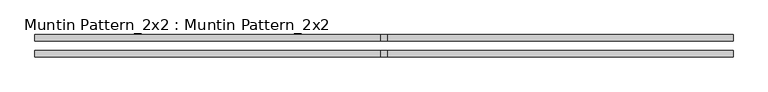
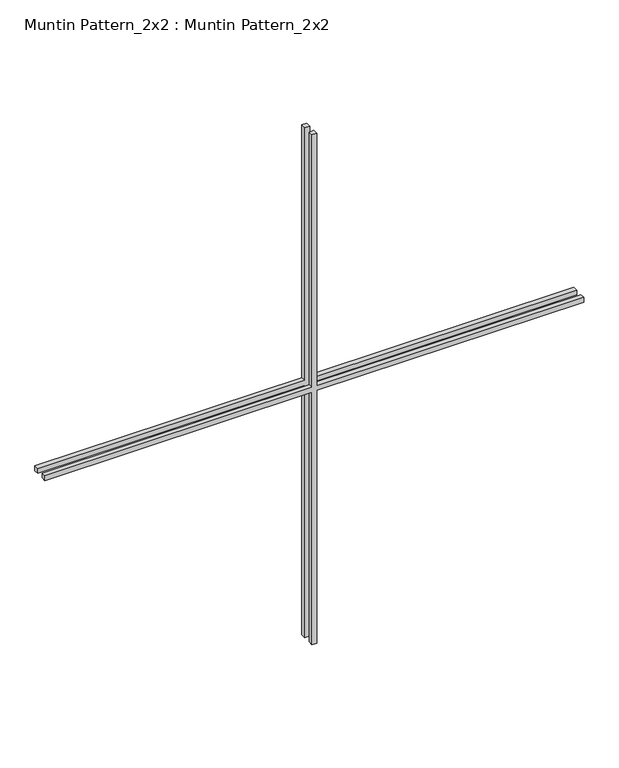
"""IFC4 building model written with IfcOpenShell, lengths in millimetres: proxy geometry, Muntin Pattern_2x2 : Muntin Pattern_2x2."""

from ifc_helpers import new_model, si_unit, frame, origin, place, context, project, spatial, polyline, outline, extrude, source, transform, mapped, element, save


def muntin_pattern_2x2_muntin_pattern_2x2_eeef18e2(model_context):
    return source(origin(), model_context, "Body", "SweptSolid", [
        extrude(outline(polyline([(698.5, -6.35), (698.5, -692.15), (685.8, -692.15), (685.8, -6.35), (0.0, -6.35), (0.0, 6.35), (685.8, 6.35), (685.8, 692.15), (698.5, 692.15), (698.5, 6.35), (1384.3, 6.35), (1384.3, -6.35), (698.5, -6.35)])), frame((0.0, 9.525, 0.0), z_axis=(0.0, 1.0, 0.0), x_axis=(0.0, 0.0, 1.0)), (0.0, 0.0, 1.0), 12.7),
        extrude(outline(polyline([(698.5, -6.35), (698.5, -692.15), (685.8, -692.15), (685.8, -6.35), (0.0, -6.35), (0.0, 6.35), (685.8, 6.35), (685.8, 692.15), (698.5, 692.15), (698.5, 6.35), (1384.3, 6.35), (1384.3, -6.35), (698.5, -6.35)])), frame((0.0, -22.225, 0.0), z_axis=(0.0, 1.0, 0.0), x_axis=(0.0, 0.0, 1.0)), (0.0, 0.0, 1.0), 12.7),
    ])


if __name__ == "__main__":
    model = new_model("IFC4")
    model_context = context("Model", 3, world=origin())
    ifc_project = project(units=[si_unit("LENGTHUNIT", "METRE", prefix="MILLI")], contexts=[model_context])
    site = spatial("IfcSite", under=ifc_project)
    building = spatial("IfcBuilding", under=site)
    placement = place(None, origin())
    muntin_pattern_2x2_muntin_pattern_2x2_shape = muntin_pattern_2x2_muntin_pattern_2x2_eeef18e2(model_context)
    element("IfcBuildingElementProxy", 1, Name="Muntin Pattern_2x2 : Muntin Pattern_2x2", ObjectType="Muntin Pattern_2x2 : Muntin Pattern_2x2", at=placement, inside=building, context=model_context, shape_type="MappedRepresentation", body=[
        mapped(muntin_pattern_2x2_muntin_pattern_2x2_shape, transform((0.0, 0.0, 0.0), x_axis=(1.0, 0.0, 0.0), y_axis=(0.0, 1.0, 0.0), z_axis=(0.0, 0.0, 1.0))),
    ])
    save(model, "model.ifc")

# Revit data of these elements
# Type "Muntin Pattern_2x2 : Muntin Pattern_2x2"
#   Width [instance default] = 4' - 0"
#   Thickness = 0' - 0 1/2"
#   Height [instance default] = 4' - 0"
#   Distance = 0' - 0 3/4"
#   Interior Material [instance default] = none
#   Exterior Material [instance default] = none
#   Default Elevation = 0
# Element 1 (IfcBuildingElementProxy, "Muntin Pattern_2x2 : Muntin Pattern_2x2")
#   Width = 4' - 6 1/2"
#   Height = 4' - 6 1/2"
#   Interior Material = Wood - Stained
#   Exterior Material = Clad - White
#   Materials on its faces: "Clad - White", "Wood - Stained"
# Materials
#   "Clad - White": class "Wood", colour RGB 242 242 238, transparency 0, Cost = 0
#   "Wood - Stained": class "Wood", colour RGB 224 178 126, transparency 0, Cost = 0
